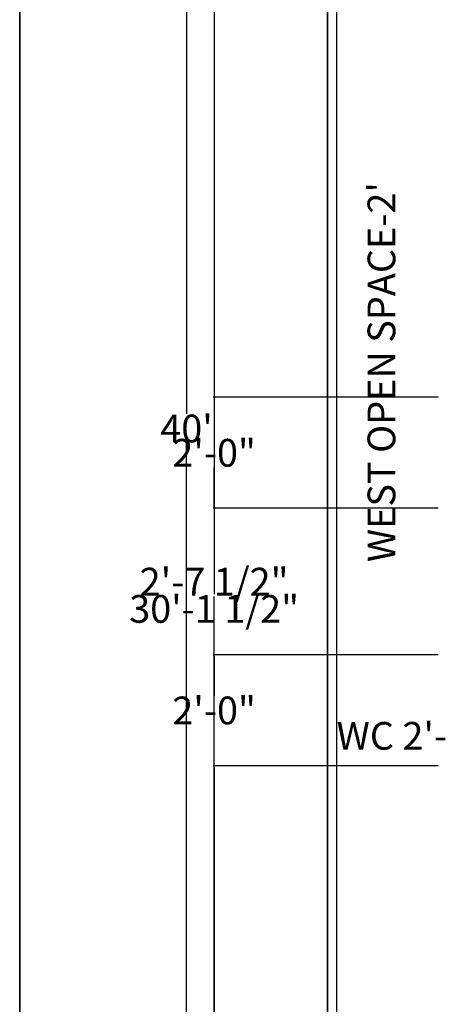
# Model space of a CAD drawing. Units: inches. Extents: x 56944 to 57417, y 173916 to 174454.
# Tile 2 of 8: x 56944 to 57034, y 174056 to 174268. Entities that reach past the tile are written whole.
import ezdxf

# ---------------------------------------------------------------- set-up
doc = ezdxf.new("R2010")
doc.units = ezdxf.units.IN
doc.header["$MEASUREMENT"] = 0
for name, color, linetype, lineweight in [('A-ANNO-DIMS', 2, 'Continuous', 18), ('A-ANNO-TEXT', 7, 'Continuous', 18), ('A-ANNO-TTLB', 7, 'Continuous', 35), ('A-SITE-WALL', 7, 'Continuous', 25), ('C-PROP', 7, 'Continuous', 35)]:
    doc.layers.add(name, color=color, linetype=linetype, lineweight=lineweight)
doc.styles.get("Standard").update_dxf_attribs({"font": 'arial.ttf'})
doc.dimstyles.get("Standard").update_dxf_attribs({"dimtxt": 6, "dimasz": 0.18, "dimexe": 0.18, "dimexo": 0.0625, "dimgap": 0.09, "dimtad": 0, "dimtih": 1, "dimtoh": 1, "dimdec": 1, "dimzin": 0, "dimdsep": 46, "dimlunit": 3, "dimtxsty": 'Standard', "dimcen": 0.09, "dimadec": 0, "dimazin": 0, "dimtfac": 1, "dimtdec": 1, "dimtofl": 0, "dimtmove": 0, "dimatfit": 3, "dimfxl": 1, "dimtolj": 1, "dimtzin": 0, "dimarcsym": 0})

# ---------------------------------------------------------------- blocks, each defined once
blk = doc.blocks.new('*D4')
at = {"layer": 'A-ANNO-DIMS', "color": 0, "lineweight": -2, "transparency": 16777216}
for p, q in [((57010.07, 174399.82), (56979.48, 174399.82)), ((56979.66, 174399.64), (56979.66, 174183.23)), ((56979.66, 173960.5), (56979.66, 174176.92)), ((57010.07, 173960.32), (56979.48, 173960.32))]:
    blk.add_line(p, q, dxfattribs=at)
at = {"layer": 'A-ANNO-DIMS', "color": 0, "transparency": 16777216}
for points in [[(56979.63, 174399.64), (56979.69, 174399.64), (56979.66, 174399.82)], [(56979.63, 173960.5), (56979.69, 173960.5), (56979.66, 173960.32)]]:
    blk.add_solid(points, dxfattribs=at)
at = {"layer": 'Defpoints', "color": 0, "transparency": 16777216}
for p in [(57010.13, 174399.82), (56979.66, 173960.32), (57010.13, 173960.32)]:
    blk.add_point(p, dxfattribs=at)
at = {"layer": 'A-ANNO-DIMS', "color": 0, "transparency": 16777216, "insert": (56979.66, 174180.07), "char_height": 6, "width": 27.5975, "attachment_point": 5}
blk.add_mtext("\\A1;40'", dxfattribs=at)
blk = doc.blocks.new('*D20')
at = {"layer": 'A-ANNO-DIMS', "color": 0, "lineweight": -2, "transparency": 16777216}
for p, q in [((57048.37, 174126.33), (57044.44, 174126.33)), ((57044.62, 174126.15), (57044.62, 174116.81)), ((57044.62, 174101.09), (57044.62, 174110.43)), ((57048.37, 174100.91), (57044.44, 174100.91))]:
    blk.add_line(p, q, dxfattribs=at)
at = {"layer": 'A-ANNO-DIMS', "color": 0, "transparency": 16777216}
for points in [[(57044.59, 174126.15), (57044.65, 174126.15), (57044.62, 174126.33)], [(57044.59, 174101.09), (57044.65, 174101.09), (57044.62, 174100.91)]]:
    blk.add_solid(points, dxfattribs=at)
at = {"layer": 'Defpoints', "color": 0, "transparency": 16777216}
for p in [(57044.62, 174126.33), (57048.43, 174126.33), (57048.43, 174100.91)]:
    blk.add_point(p, dxfattribs=at)
at = {"layer": 'A-ANNO-DIMS', "color": 0, "transparency": 16777216, "insert": (57044.62, 174113.62), "char_height": 6, "attachment_point": 5}
blk.add_mtext('\\A1;WC 2\'-1 1/2" TYP.', dxfattribs=at)
blk = doc.blocks.new('*D37')
at = {"layer": 'A-ANNO-DIMS', "color": 0, "lineweight": -2, "transparency": 16777216}
for p, q in [((57034.07, 174321.82), (56985.45, 174321.82)), ((56985.63, 174321.64), (56985.63, 174144.27)), ((56985.63, 173960.5), (56985.63, 174137.88)), ((57034.07, 173960.32), (56985.45, 173960.32))]:
    blk.add_line(p, q, dxfattribs=at)
at = {"layer": 'A-ANNO-DIMS', "color": 0, "transparency": 16777216}
for points in [[(56985.6, 174321.64), (56985.66, 174321.64), (56985.63, 174321.82)], [(56985.6, 173960.5), (56985.66, 173960.5), (56985.63, 173960.32)]]:
    blk.add_solid(points, dxfattribs=at)
at = {"layer": 'Defpoints', "color": 0, "transparency": 16777216}
for p in [(56985.63, 174321.82), (57034.13, 174321.82), (57034.13, 173960.32)]:
    blk.add_point(p, dxfattribs=at)
at = {"layer": 'A-ANNO-DIMS', "color": 0, "transparency": 16777216, "insert": (56985.63, 174141.07), "char_height": 6, "attachment_point": 5}
blk.add_mtext('\\A1;30\'-1 1/2"', dxfattribs=at)
blk = doc.blocks.new('*D59')
at = {"layer": 'A-ANNO-DIMS', "color": 0, "lineweight": -2, "transparency": 16777216}
for p, q in [((57034.07, 174186.82), (56985.45, 174186.82)), ((56985.63, 174186.64), (56985.63, 174177.98)), ((56985.63, 174163), (56985.63, 174171.67)), ((57034.07, 174162.82), (56985.45, 174162.82))]:
    blk.add_line(p, q, dxfattribs=at)
at = {"layer": 'A-ANNO-DIMS', "color": 0, "transparency": 16777216}
for points in [[(56985.6, 174186.64), (56985.66, 174186.64), (56985.63, 174186.82)], [(56985.6, 174163), (56985.66, 174163), (56985.63, 174162.82)]]:
    blk.add_solid(points, dxfattribs=at)
at = {"layer": 'Defpoints', "color": 0, "transparency": 16777216}
for p in [(56985.63, 174186.82), (57034.13, 174186.82), (57034.13, 174162.82)]:
    blk.add_point(p, dxfattribs=at)
at = {"layer": 'A-ANNO-DIMS', "color": 0, "transparency": 16777216, "insert": (56985.63, 174174.82), "char_height": 6, "attachment_point": 5}
blk.add_mtext('\\A1;2\'-0"', dxfattribs=at)
blk = doc.blocks.new('*D60')
at = {"layer": 'A-ANNO-DIMS', "color": 0, "lineweight": -2, "transparency": 16777216}
for p, q in [((57034.07, 174131.11), (56985.45, 174131.11)), ((56985.63, 174130.93), (56985.63, 174122.26)), ((56985.63, 174107.29), (56985.63, 174115.95)), ((57034.07, 174107.11), (56985.45, 174107.11))]:
    blk.add_line(p, q, dxfattribs=at)
at = {"layer": 'A-ANNO-DIMS', "color": 0, "transparency": 16777216}
for points in [[(56985.6, 174130.93), (56985.66, 174130.93), (56985.63, 174131.11)], [(56985.6, 174107.29), (56985.66, 174107.29), (56985.63, 174107.11)]]:
    blk.add_solid(points, dxfattribs=at)
at = {"layer": 'Defpoints', "color": 0, "transparency": 16777216}
for p in [(56985.63, 174131.11), (57034.13, 174131.11), (57034.13, 174107.11)]:
    blk.add_point(p, dxfattribs=at)
at = {"layer": 'A-ANNO-DIMS', "color": 0, "transparency": 16777216, "insert": (56985.63, 174119.11), "char_height": 6, "attachment_point": 5}
blk.add_mtext('\\A1;2\'-0"', dxfattribs=at)
blk = doc.blocks.new('*D61')
at = {"layer": 'A-ANNO-DIMS', "color": 0, "lineweight": -2, "transparency": 16777216}
for p, q in [((57034.07, 174162.82), (56985.45, 174162.82)), ((56985.63, 174162.64), (56985.63, 174150.16)), ((56985.63, 174131.29), (56985.63, 174143.77)), ((57034.07, 174131.11), (56985.45, 174131.11))]:
    blk.add_line(p, q, dxfattribs=at)
at = {"layer": 'A-ANNO-DIMS', "color": 0, "transparency": 16777216}
for points in [[(56985.6, 174162.64), (56985.66, 174162.64), (56985.63, 174162.82)], [(56985.6, 174131.29), (56985.66, 174131.29), (56985.63, 174131.11)]]:
    blk.add_solid(points, dxfattribs=at)
at = {"layer": 'Defpoints', "color": 0, "transparency": 16777216}
for p in [(56985.63, 174162.82), (57034.13, 174162.82), (57034.13, 174131.11)]:
    blk.add_point(p, dxfattribs=at)
at = {"layer": 'A-ANNO-DIMS', "color": 0, "transparency": 16777216, "insert": (56985.63, 174146.96), "char_height": 6, "attachment_point": 5}
blk.add_mtext('\\A1;2\'-7 1/2"', dxfattribs=at)
blk = doc.blocks.new('*D62')
at = {"layer": 'A-ANNO-DIMS', "color": 0, "lineweight": -2, "transparency": 16777216}
for p, q in [((57034.07, 174107.11), (56985.45, 174107.11)), ((56985.63, 174106.93), (56985.63, 174036.87)), ((56985.63, 173960.5), (56985.63, 174030.56)), ((57034.07, 173960.32), (56985.45, 173960.32))]:
    blk.add_line(p, q, dxfattribs=at)
at = {"layer": 'A-ANNO-DIMS', "color": 0, "transparency": 16777216}
for points in [[(56985.6, 174106.93), (56985.66, 174106.93), (56985.63, 174107.11)], [(56985.6, 173960.5), (56985.66, 173960.5), (56985.63, 173960.32)]]:
    blk.add_solid(points, dxfattribs=at)
at = {"layer": 'Defpoints', "color": 0, "transparency": 16777216}
for p in [(57034.13, 174107.11), (56985.63, 173960.32), (57034.13, 173960.32)]:
    blk.add_point(p, dxfattribs=at)
at = {"layer": 'A-ANNO-DIMS', "color": 0, "transparency": 16777216, "insert": (56985.63, 174033.71), "char_height": 6, "attachment_point": 5}
blk.add_mtext('\\A1;12\'-3"', dxfattribs=at)

msp = doc.modelspace()

# ---------------------------------------------------------------- linework, layer by layer
at = {"layer": 'A-ANNO-TTLB'}
msp.add_lwpolyline([(56943.57, 174453.61), (57416.55, 174453.61), (57416.55, 173915.6), (56943.57, 173915.6)], close=True, dxfattribs=at)
at = {"layer": 'A-SITE-WALL'}
msp.add_line((57012.13, 174397.82), (57012.13, 173960.32), dxfattribs=at)
at = {"layer": 'C-PROP'}
msp.add_line((57010.13, 174399.82), (57010.13, 173960.32), dxfattribs=at)

# ---------------------------------------------------------------- texts
at = {"layer": 'A-ANNO-TEXT', "insert": (57018.83, 174151.18), "char_height": 6, "attachment_point": 1, "rotation": 90}
msp.add_mtext_dynamic_manual_height_columns("WEST OPEN SPACE-2'", width=155.7027, gutter_width=1, heights=[0], dxfattribs=at)

# ---------------------------------------------------------------- dimensions: what is measured, and where the dimension line sits
at = {"layer": 'A-ANNO-DIMS'}
for base, p1, p2, text, override, picture, middle in [((56979.66, 173960.32), (57010.13, 174399.82), (57010.13, 173960.32), "40'", {"dimclrd": 0, "dimclre": 0, "dimclrt": 0}, '*D4', (56979.66, 174180.07)), ((57044.62, 174126.33), (57048.43, 174100.91), (57048.43, 174126.33), 'WC <> TYP.', {"dimdec": 1, "dimlfac": 1, "dimrnd": 0, "dimzin": 1, "dimdsep": 46, "dimlunit": 4, "dimfrac": 2}, '*D20', (57044.62, 174113.62))]:
    dim = msp.add_linear_dim(base=base, p1=p1, p2=p2, angle=90, text=text, dimstyle='Standard', override=override, dxfattribs=at)
    dim.commit()
    dim.dimension.update_dxf_attribs({"geometry": picture, "text_midpoint": middle})
for base, p1, p2, picture, middle in [((56985.63, 174321.82), (57034.13, 173960.32), (57034.13, 174321.82), '*D37', (56985.63, 174141.07)), ((56985.63, 174186.82), (57034.13, 174162.82), (57034.13, 174186.82), '*D59', (56985.63, 174174.82)), ((56985.63, 174162.82), (57034.13, 174131.11), (57034.13, 174162.82), '*D61', (56985.63, 174146.96)), ((56985.63, 174131.11), (57034.13, 174107.11), (57034.13, 174131.11), '*D60', (56985.63, 174119.11)), ((56985.63, 173960.32), (57034.13, 174107.11), (57034.13, 173960.32), '*D62', (56985.63, 174033.71))]:
    dim = msp.add_linear_dim(base=base, p1=p1, p2=p2, angle=90, dimstyle='Standard', override={"dimdec": 1, "dimlfac": 1, "dimrnd": 0, "dimzin": 1, "dimdsep": 46, "dimlunit": 4, "dimfrac": 2}, dxfattribs=at)
    dim.commit()
    dim.dimension.update_dxf_attribs({"geometry": picture, "text_midpoint": middle})

doc.saveas('drawing.dxf')
